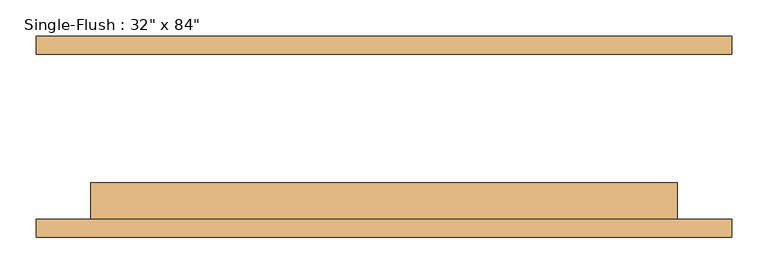
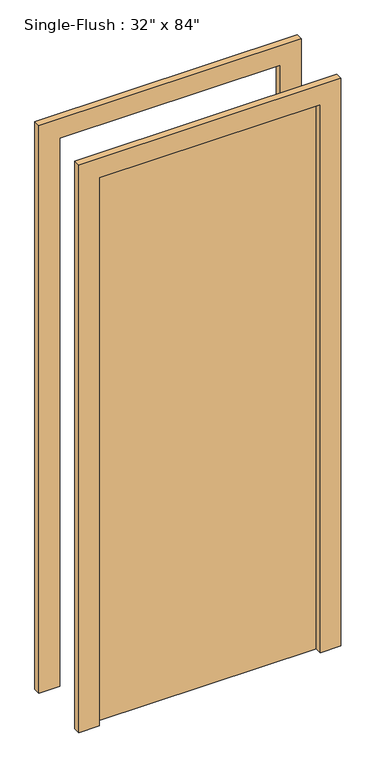
"""IFC4 building model written with IfcOpenShell, lengths in millimetres: door geometry."""

from ifc_helpers import new_model, si_unit, frame, origin, origin_with_axes, place, context, project, spatial, polyline, outline, extrude, source, transform, mapped, element, save


def door_7b345704(model_context):
    return source(origin(), model_context, "Body", "SweptSolid", [
        extrude(outline(polyline([(2209.8, -482.6), (0.0, -482.6), (0.0, -406.4), (2133.6, -406.4), (2133.6, 406.4), (0.0, 406.4), (0.0, 482.6), (2209.8, 482.6), (2209.8, -482.6)])), frame((0.0, -139.7, 0.0), z_axis=(0.0, 1.0, 0.0), x_axis=(0.0, 0.0, 1.0)), (0.0, 0.0, 1.0), 25.4),
        extrude(outline(polyline([(2209.8, 482.6), (2209.8, -482.6), (0.0, -482.6), (0.0, -406.4), (2133.6, -406.4), (2133.6, 406.4), (0.0, 406.4), (0.0, 482.6), (2209.8, 482.6)])), frame((0.0, 114.3, 0.0), z_axis=(0.0, 1.0, 0.0), x_axis=(0.0, 0.0, 1.0)), (0.0, 0.0, 1.0), 25.4),
        extrude(outline(polyline([(406.4, -63.5), (406.4, -114.3), (-406.4, -114.3), (-406.4, -63.5), (406.4, -63.5)])), origin_with_axes(), (0.0, 0.0, 1.0), 2133.6),
    ])


if __name__ == "__main__":
    model = new_model("IFC4")
    model_context = context("Model", 3, world=origin())
    ifc_project = project(units=[si_unit("LENGTHUNIT", "METRE", prefix="MILLI")], contexts=[model_context])
    site = spatial("IfcSite", under=ifc_project)
    building = spatial("IfcBuilding", under=site)
    placement = place(None, origin())
    door_shape = door_7b345704(model_context)
    element("IfcDoor", 1, ObjectType="Single-Flush : 32\" x 84\"", at=placement, inside=building, context=model_context, shape_type="MappedRepresentation", body=[
        mapped(door_shape, transform((0.0, 0.0, 0.0), x_axis=(1.0, 0.0, 0.0), y_axis=(0.0, 1.0, 0.0), z_axis=(0.0, 0.0, 1.0))),
    ])
    save(model, "model.ifc")

# Revit data of these elements
# Type "Single-Flush : 32\" x 84\""
#   Type Mark = "3"
#   Construction Type Id = "MDOOR"
#   Assembly Code = "C1020"
#   Analytic Construction = "Metal"
#   Thickness = 0' - 2"
#   Heat Transfer Coefficient (U) = 0.651978 BTU/(h·ft²·°F)
#   Height = 7' - 0"
#   Trim Projection Ext = 0' - 1"
#   Trim Projection Int = 0' - 1"
#   Trim Width = 0' - 3"
#   Width = 2' - 8"
#   Define Thermal Properties by = 1
#   Define Thermal Properties by = 1
#   Door Material = Door - Panel
#   Frame Material = Door - Frame
#   Visual Light Transmittance = 0
#   Solar Heat Gain Coefficient = 0
#   Function = (empty or 0)
#   Wall Closure = (empty or 0)
# Element 1 (IfcDoor, "Single-Flush : 32\" x 84\"")
#   Materials on its faces: "Door - Frame", "Door - Panel"
# Materials
#   "Door - Panel": class "Wood", colour RGB 210 159 95, transparency 0, Cost = 0
#   "Door - Frame": colour RGB 118 70 51, transparency 0, Cost = 0
